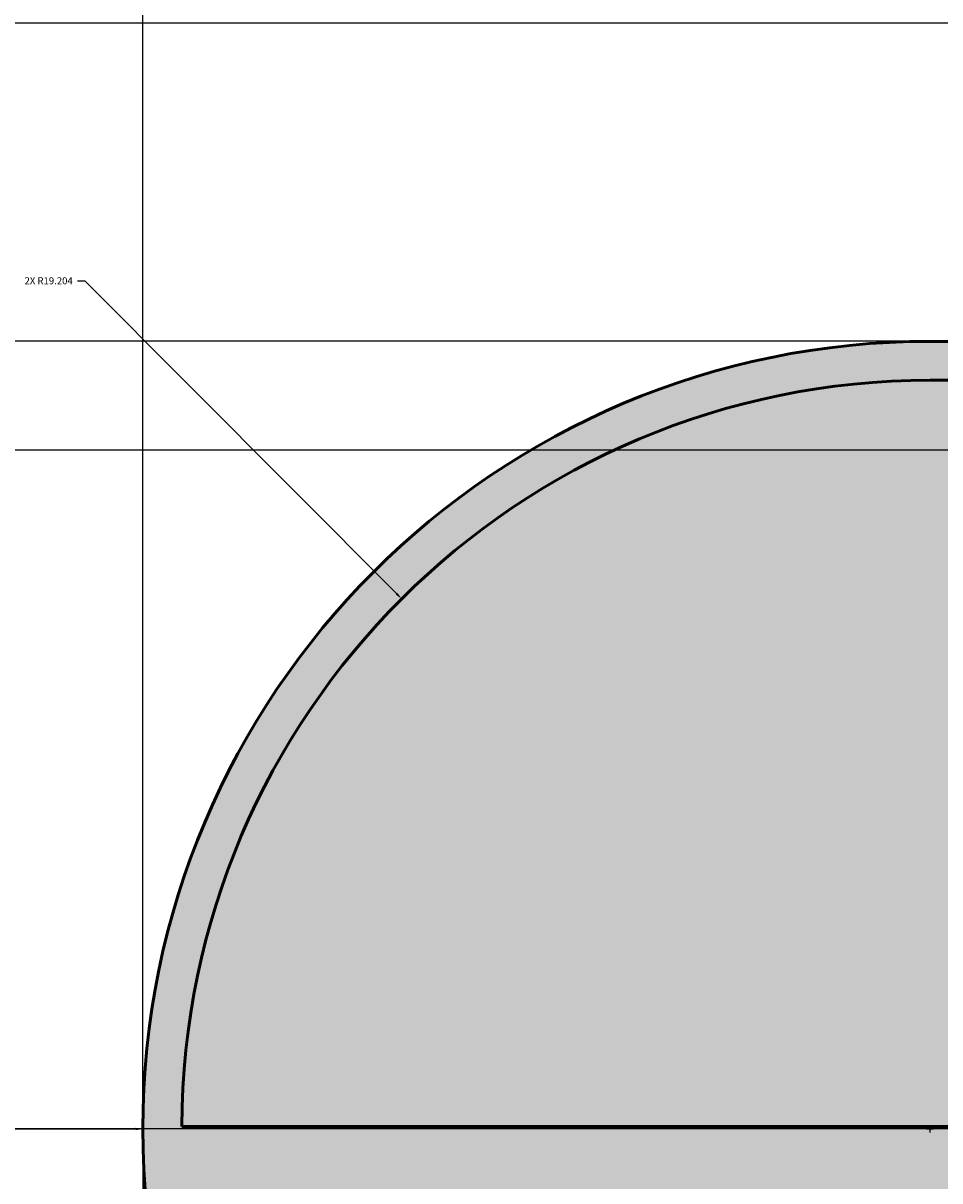
# Model space of a CAD drawing. Units: inches. Extents: x -12 to 334, y -10 to 186.
# Tile 7 of 77: x 0 to 24, y 79 to 109. Entities that reach past the tile are written whole.
import ezdxf

# ---------------------------------------------------------------- set-up
doc = ezdxf.new("R2010")
doc.units = ezdxf.units.IN
doc.header["$MEASUREMENT"] = 0
for name, color, linetype, lineweight in [('M-DIMS', 2, 'Continuous', 18), ('M-EQPM', 7, 'Continuous', 50), ('M-EQPM-PATT', 8, 'Continuous', 18)]:
    doc.layers.add(name, color=color, linetype=linetype, lineweight=lineweight)
doc.styles.get("Standard").update_dxf_attribs({"font": 'arial.ttf'})
doc.dimstyles.get("Standard").update_dxf_attribs({"dimtxt": 0.18, "dimasz": 0.18, "dimexe": 0.18, "dimexo": 0.0625, "dimgap": 0.09, "dimtad": 0, "dimtih": 1, "dimtoh": 1, "dimdec": 4, "dimzin": 0, "dimdsep": 46, "dimtxsty": 'Standard', "dimcen": 0.09, "dimadec": 0, "dimazin": 0, "dimtfac": 1, "dimtdec": 4, "dimtofl": 0, "dimtmove": 0, "dimatfit": 3, "dimfxl": 1, "dimtolj": 1, "dimtzin": 0, "dimarcsym": 0})

# ---------------------------------------------------------------- blocks, each defined once
blk = doc.blocks.new('*D1')
at = {"layer": 'Defpoints', "color": 0, "transparency": 16777216}
for p in [(281.426, 91.899), (3.376, 80.692), (281.426, 14.304)]:
    blk.add_point(p, dxfattribs=at)
at = {"layer": 'M-DIMS', "color": 0, "lineweight": -2, "transparency": 16777216}
for p, q in [((281.426, 91.836), (281.426, 14.124)), ((3.376, 80.629), (3.376, 14.124)), ((3.556, 14.304), (141.935, 14.304)), ((281.246, 14.304), (142.867, 14.304))]:
    blk.add_line(p, q, dxfattribs=at)
at = {"layer": 'M-DIMS', "color": 0, "transparency": 16777216}
for points in [[(3.556, 14.334), (3.556, 14.274), (3.376, 14.304)], [(281.246, 14.334), (281.246, 14.274), (281.426, 14.304)]]:
    blk.add_solid(points, dxfattribs=at)
at = {"layer": 'M-DIMS', "color": 0, "transparency": 16777216, "insert": (142.401, 14.304), "char_height": 0.18, "attachment_point": 5}
blk.add_mtext('\\A1;278.05', dxfattribs=at)
blk = doc.blocks.new('*D2')
at = {"layer": 'Defpoints', "color": 0, "transparency": 16777216}
for p in [(32.1, 169.385), (32.1, 127.708), (3.376, 80.692)]:
    blk.add_point(p, dxfattribs=at)
at = {"layer": 'M-DIMS', "color": 0, "lineweight": -2, "transparency": 16777216}
for p, q in [((3.376, 80.754), (3.376, 169.565)), ((3.556, 169.385), (17.274, 169.385)), ((31.92, 169.385), (18.203, 169.385)), ((32.1, 127.77), (32.1, 169.565))]:
    blk.add_line(p, q, dxfattribs=at)
at = {"layer": 'M-DIMS', "color": 0, "transparency": 16777216}
for points in [[(3.556, 169.415), (3.556, 169.355), (3.376, 169.385)], [(31.92, 169.415), (31.92, 169.355), (32.1, 169.385)]]:
    blk.add_solid(points, dxfattribs=at)
at = {"layer": 'M-DIMS', "color": 0, "transparency": 16777216, "insert": (17.738, 169.385), "char_height": 0.18, "attachment_point": 5}
blk.add_mtext('\\A1;28.724', dxfattribs=at)
blk = doc.blocks.new('*D7')
at = {"layer": 'Defpoints', "color": 0, "transparency": 16777216}
for p in [(-11.174, 100.896), (23.581, 100.896), (23.581, 60.487)]:
    blk.add_point(p, dxfattribs=at)
at = {"layer": 'M-DIMS', "color": 0, "lineweight": -2, "transparency": 16777216}
for p, q in [((23.518, 100.896), (-11.354, 100.896)), ((-11.174, 100.716), (-11.174, 80.873)), ((-11.174, 60.667), (-11.174, 80.51)), ((23.518, 60.487), (-11.354, 60.487))]:
    blk.add_line(p, q, dxfattribs=at)
at = {"layer": 'M-DIMS', "color": 0, "transparency": 16777216}
for points in [[(-11.204, 100.716), (-11.144, 100.716), (-11.174, 100.896)], [(-11.204, 60.667), (-11.144, 60.667), (-11.174, 60.487)]]:
    blk.add_solid(points, dxfattribs=at)
at = {"layer": 'M-DIMS', "color": 0, "transparency": 16777216, "insert": (-11.174, 80.692), "char_height": 0.18, "attachment_point": 5}
blk.add_mtext('\\A1;40.41', dxfattribs=at)
blk = doc.blocks.new('*D8')
at = {"layer": 'Defpoints', "color": 0, "transparency": 16777216}
for p in [(-11.174, 127.708), (32.1, 127.708), (23.581, 100.896)]:
    blk.add_point(p, dxfattribs=at)
at = {"layer": 'M-DIMS', "color": 0, "lineweight": -2, "transparency": 16777216}
for p, q in [((32.038, 127.708), (-11.354, 127.708)), ((-11.174, 127.528), (-11.174, 114.484)), ((-11.174, 101.076), (-11.174, 114.12)), ((23.518, 100.896), (-11.354, 100.896))]:
    blk.add_line(p, q, dxfattribs=at)
at = {"layer": 'M-DIMS', "color": 0, "transparency": 16777216}
for points in [[(-11.204, 127.528), (-11.144, 127.528), (-11.174, 127.708)], [(-11.204, 101.076), (-11.144, 101.076), (-11.174, 100.896)]]:
    blk.add_solid(points, dxfattribs=at)
at = {"layer": 'M-DIMS', "color": 0, "transparency": 16777216, "insert": (-11.174, 114.302), "char_height": 0.18, "attachment_point": 5}
blk.add_mtext('\\A1;26.81', dxfattribs=at)
blk = doc.blocks.new('*D14')
at = {"layer": 'Defpoints', "color": 0, "transparency": 16777216}
for p in [(63.5, 109.058), (-11.174, 49.45), (64.207, 49.45)]:
    blk.add_point(p, dxfattribs=at)
at = {"layer": 'M-DIMS', "color": 0, "lineweight": -2, "transparency": 16777216}
for p, q in [((63.438, 109.058), (-11.354, 109.058)), ((-11.174, 108.878), (-11.174, 79.436)), ((-11.174, 49.63), (-11.174, 79.072)), ((64.144, 49.45), (-11.354, 49.45))]:
    blk.add_line(p, q, dxfattribs=at)
at = {"layer": 'M-DIMS', "color": 0, "transparency": 16777216}
for points in [[(-11.204, 108.878), (-11.144, 108.878), (-11.174, 109.058)], [(-11.204, 49.63), (-11.144, 49.63), (-11.174, 49.45)]]:
    blk.add_solid(points, dxfattribs=at)
at = {"layer": 'M-DIMS', "color": 0, "transparency": 16777216, "insert": (-11.174, 79.254), "char_height": 0.18, "attachment_point": 5}
blk.add_mtext('\\A1;59.61', dxfattribs=at)
blk = doc.blocks.new('*D35')
at = {"layer": 'Defpoints', "color": 0, "transparency": 16777216}
for p in [(216.428, 98.108), (-11.174, 61.105), (216.428, 61.105)]:
    blk.add_point(p, dxfattribs=at)
at = {"layer": 'M-DIMS', "color": 0, "lineweight": -2, "transparency": 16777216}
for p, q in [((216.365, 98.108), (-11.354, 98.108)), ((-11.174, 97.928), (-11.174, 79.788)), ((-11.174, 61.285), (-11.174, 79.424)), ((216.365, 61.105), (-11.354, 61.105))]:
    blk.add_line(p, q, dxfattribs=at)
at = {"layer": 'M-DIMS', "color": 0, "transparency": 16777216}
for points in [[(-11.204, 97.928), (-11.144, 97.928), (-11.174, 98.108)], [(-11.204, 61.285), (-11.144, 61.285), (-11.174, 61.105)]]:
    blk.add_solid(points, dxfattribs=at)
at = {"layer": 'M-DIMS', "color": 0, "transparency": 16777216, "insert": (-11.174, 79.606), "char_height": 0.18, "attachment_point": 5}
blk.add_mtext('\\A1;37', dxfattribs=at)
blk = doc.blocks.new('*D39')
at = {"layer": 'Defpoints', "color": 0, "transparency": 16777216}
for p in [(279.726, 80.692), (-11.174, 45.854), (269.381, 45.854)]:
    blk.add_point(p, dxfattribs=at)
at = {"layer": 'M-DIMS', "color": 0, "lineweight": -2, "transparency": 16777216}
for p, q in [((279.664, 80.692), (-11.354, 80.692)), ((-11.174, 80.512), (-11.174, 63.455)), ((-11.174, 46.034), (-11.174, 63.091)), ((269.318, 45.854), (-11.354, 45.854))]:
    blk.add_line(p, q, dxfattribs=at)
at = {"layer": 'M-DIMS', "color": 0, "transparency": 16777216}
for points in [[(-11.204, 80.512), (-11.144, 80.512), (-11.174, 80.692)], [(-11.204, 46.034), (-11.144, 46.034), (-11.174, 45.854)]]:
    blk.add_solid(points, dxfattribs=at)
at = {"layer": 'M-DIMS', "color": 0, "transparency": 16777216, "insert": (-11.174, 63.273), "char_height": 0.18, "attachment_point": 5}
blk.add_mtext('\\A1;34.84', dxfattribs=at)
blk = doc.blocks.new('*D42')
at = {"layer": 'Defpoints', "color": 0, "transparency": 16777216}
for p in [(3.376, 80.69), (23.581, 80.692)]:
    blk.add_point(p, dxfattribs=at)
at = {"layer": 'M-DIMS', "color": 0, "lineweight": -2, "transparency": 16777216}
for p, q in [((23.581, 80.602), (23.581, 80.782)), ((-8.746, 80.689), (3.196, 80.69)), ((23.491, 80.692), (23.671, 80.692))]:
    blk.add_line(p, q, dxfattribs=at)
at = {"layer": 'M-DIMS', "color": 0, "transparency": 16777216}
blk.add_solid([(3.196, 80.72), (3.196, 80.66), (3.376, 80.69)], dxfattribs=at)
at = {"layer": 'M-DIMS', "color": 0, "transparency": 16777216, "insert": (-9.296, 80.689), "char_height": 0.18, "attachment_point": 5}
blk.add_mtext('\\A1;R20.204', dxfattribs=at)
blk = doc.blocks.new('*D44')
at = {"layer": 'Defpoints', "color": 0, "transparency": 16777216}
for p in [(10.02, 94.29), (23.581, 80.692)]:
    blk.add_point(p, dxfattribs=at)
at = {"layer": 'M-DIMS', "color": 0, "lineweight": -2, "transparency": 16777216}
for p, q in [((1.704, 102.449), (1.884, 102.449)), ((1.884, 102.449), (9.893, 94.417)), ((23.581, 80.602), (23.581, 80.782)), ((23.491, 80.692), (23.671, 80.692))]:
    blk.add_line(p, q, dxfattribs=at)
at = {"layer": 'M-DIMS', "color": 0, "transparency": 16777216}
blk.add_solid([(9.914, 94.438), (9.872, 94.396), (10.02, 94.29)], dxfattribs=at)
at = {"layer": 'M-DIMS', "color": 0, "transparency": 16777216, "insert": (0.959, 102.449), "char_height": 0.18, "attachment_point": 5}
blk.add_mtext('\\A1;2X R19.204', dxfattribs=at)

msp = doc.modelspace()

# ---------------------------------------------------------------- hatches: boundary and pattern name
at = {"layer": 'M-EQPM-PATT'}
h = msp.add_hatch(color=256, dxfattribs=at)
h.set_gradient(color1=(99, 100, 102), color2=(99, 100, 102), tint=1)
h.paths.add_polyline_path([(4.3766, 80.754, -0.4132606), (23.5807, 99.8958), (37.1002, 99.8958), (37.1002, 127.7078), (32.1002, 127.7078), (32.1002, 125.2078), (36.1002, 125.2078), (36.1002, 100.8958), (23.5807, 100.8958, 1), (23.5807, 60.4872), (36.1002, 60.4872), (36.1002, 36.1752), (32.1002, 36.1752), (32.1002, 33.6752), (37.1002, 33.6752), (37.1002, 61.4872), (23.5807, 61.4872, -0.384914), (4.4744, 78.754), (72.9244, 78.754), (72.9244, 69.6117), (75.9244, 69.6117), (75.9244, 89.8963), (72.9244, 89.8963), (72.9244, 80.754)])
h.paths.add_polyline_path([(54.1002, 125.2078), (58.1002, 125.2078), (58.1002, 127.7078), (53.1002, 127.7078), (53.1002, 99.8958), (64.5, 99.8958), (64.5, 109.0583), (63.5, 109.0583), (63.5, 100.8958), (54.1002, 100.8958)], flags=17)
h.paths.add_polyline_path([(53.1002, 33.6752), (58.1002, 33.6752), (58.1002, 36.1752), (54.1002, 36.1752), (54.1002, 60.4872), (64.2068, 60.4872), (64.2068, 49.4497), (87.8879, 49.4497), (87.8879, 55.3205), (104.8919, 55.3205), (104.8919, 30.8541), (99.8919, 30.8541), (99.8919, 28.8541), (105.8919, 28.8541), (105.8919, 56.3205), (87.8879, 56.3205), (87.8879, 63.6117), (86.8879, 63.6117), (86.8879, 50.4497), (65.0061, 50.4497), (65.0061, 63.6117), (64.5, 63.6117), (64.5, 61.4872), (53.1002, 61.4872)])
h.paths.add_polyline_path([(121.8919, 28.8541), (121.8919, 30.8541), (116.8919, 30.8541), (116.8919, 45.8541), (209.6965, 45.8541), (209.9204, 46.8541), (115.8919, 46.8541), (115.8919, 28.8541)])
h.paths.add_polyline_path([(221.5761, 32.8541), (216.5761, 32.8541), (216.5761, 30.8541), (222.5761, 30.8541), (222.5761, 46.8541), (209.9204, 46.8541), (209.6965, 45.8541), (221.5761, 45.8541)])
h.paths.add_polyline_path([(233.5761, 45.8541), (249.8485, 45.8541), (249.3759, 46.8541), (232.5761, 46.8541), (232.5761, 30.8541), (238.5761, 30.8541), (238.5761, 32.8541), (233.5761, 32.8541)])
h = msp.add_hatch(color=256, dxfattribs=at)
h.set_gradient(color1=(205, 32, 39), color2=(205, 32, 39), tint=1)
h.paths.add_polyline_path([(64.5, 80.754), (64.5, 89.8963), (226.6083, 89.8963, -1), (226.6083, 69.6117), (64.5, 69.6117), (64.5, 78.754), (4.4744, 78.754, 0.384914), (23.5807, 61.4872), (37.1002, 61.4872), (37.1002, 33.6752), (53.1002, 33.6752), (53.1002, 61.4872), (64.5, 61.4872), (64.5, 63.6117), (226.6083, 63.6117, 1), (226.6083, 95.8963), (64.5, 95.8963), (64.5, 99.8958), (53.1002, 99.8958), (53.1002, 127.7078), (37.1002, 127.7078), (37.1002, 99.8958), (23.5807, 99.8958, 0.4132606), (4.3766, 80.754)])
h.paths.add_polyline_path([(64.5, 91.8963), (64.5, 93.8963), (226.6083, 93.8963, -1), (226.6083, 65.6117), (64.5, 65.6117), (64.5, 67.6117), (226.6083, 67.6117, 1), (226.6083, 91.8963)], flags=16)

# ---------------------------------------------------------------- linework, layer by layer
at = {"layer": 'M-EQPM'}
msp.add_line((72.9244, 80.754), (4.3766, 80.754), dxfattribs=at)
for points in [[(36.1002, 60.4872), (23.5807, 60.4872, -1), (23.5807, 100.8958), (36.1002, 100.8958)], [(4.3766, 80.754, -0.4132606), (23.5807, 99.8958), (37.1002, 99.8958)]]:
    msp.add_lwpolyline(points, format="xyb", dxfattribs=at)

# ---------------------------------------------------------------- dimensions: what is measured, and where the dimension line sits
at = {"layer": 'M-DIMS'}
for base, p2, override, picture, middle in [((32.1002, 169.3845), (32.1002, 127.7078), {"dimdec": 3, "dimlfac": 1, "dimrnd": 0, "dimzin": 0, "dimdsep": 46, "dimlunit": 2}, '*D2', (17.7383, 169.3845)), ((281.4256, 14.3041), (281.4256, 91.8988), {"dimdec": 2, "dimlfac": 1, "dimrnd": 0, "dimzin": 0, "dimdsep": 46, "dimlunit": 2}, '*D1', (142.401, 14.3041))]:
    dim = msp.add_linear_dim(base=base, p1=(3.3764, 80.6915), p2=p2, dimstyle='Standard', override=override, dxfattribs=at)
    dim.commit()
    dim.dimension.update_dxf_attribs({"geometry": picture, "text_midpoint": middle})
for base, p1, p2, override, picture, middle in [((-11.1736, 127.7078), (23.5807, 100.8958), (32.1002, 127.7078), {"dimdec": 2, "dimlfac": 1, "dimrnd": 0, "dimzin": 0, "dimdsep": 46, "dimlunit": 2}, '*D8', (-11.1735, 114.3018)), ((-11.1736, 49.4497), (63.5, 109.0583), (64.2068, 49.4497), {"dimdec": 2, "dimlfac": 1, "dimrnd": 0, "dimzin": 0, "dimdsep": 46, "dimlunit": 2}, '*D14', (-11.1735, 79.254)), ((-11.1736, 100.8958), (23.5807, 60.4872), (23.5807, 100.8958), {"dimdec": 2, "dimlfac": 1, "dimrnd": 0, "dimzin": 0, "dimdsep": 46, "dimlunit": 2}, '*D7', (-11.1735, 80.6915)), ((-11.1736, 61.1045), (216.4278, 98.1081), (216.4278, 61.1045), {"dimdec": 0, "dimlfac": 1, "dimrnd": 0, "dimzin": 0, "dimdsep": 46, "dimlunit": 2}, '*D35', (-11.1735, 79.6063)), ((-11.1736, 45.8541), (279.7263, 80.6915), (269.3808, 45.8541), {"dimdec": 2, "dimlfac": 1, "dimrnd": 0, "dimzin": 0, "dimdsep": 46, "dimlunit": 2}, '*D39', (-11.1735, 63.2728))]:
    dim = msp.add_linear_dim(base=base, p1=p1, p2=p2, angle=90, dimstyle='Standard', override=override, dxfattribs=at)
    dim.commit()
    dim.dimension.update_dxf_attribs({"geometry": picture, "text_midpoint": middle})
dim = msp.add_radius_dim(center=(23.5807, 80.6915), mpoint=(10.0201, 94.2899), text='2X <>', dimstyle='Standard', override={"dimdec": 3, "dimlfac": 1, "dimrnd": 0, "dimzin": 0, "dimdsep": 46, "dimlunit": 2}, dxfattribs=at)
dim.commit()
dim.dimension.update_dxf_attribs({"geometry": '*D44', "text_midpoint": (0.9595, 102.4489), "dimtype": 164})
dim = msp.add_radius_dim(center=(23.5807, 80.6915), mpoint=(3.3764, 80.69), dimstyle='Standard', override={"dimdec": 3, "dimlfac": 1, "dimrnd": 0, "dimzin": 0, "dimdsep": 46, "dimlunit": 2}, dxfattribs=at)
dim.commit()
dim.dimension.update_dxf_attribs({"geometry": '*D42', "text_midpoint": (-8.7461, 80.6891), "dimtype": 164})

doc.saveas('drawing.dxf')
